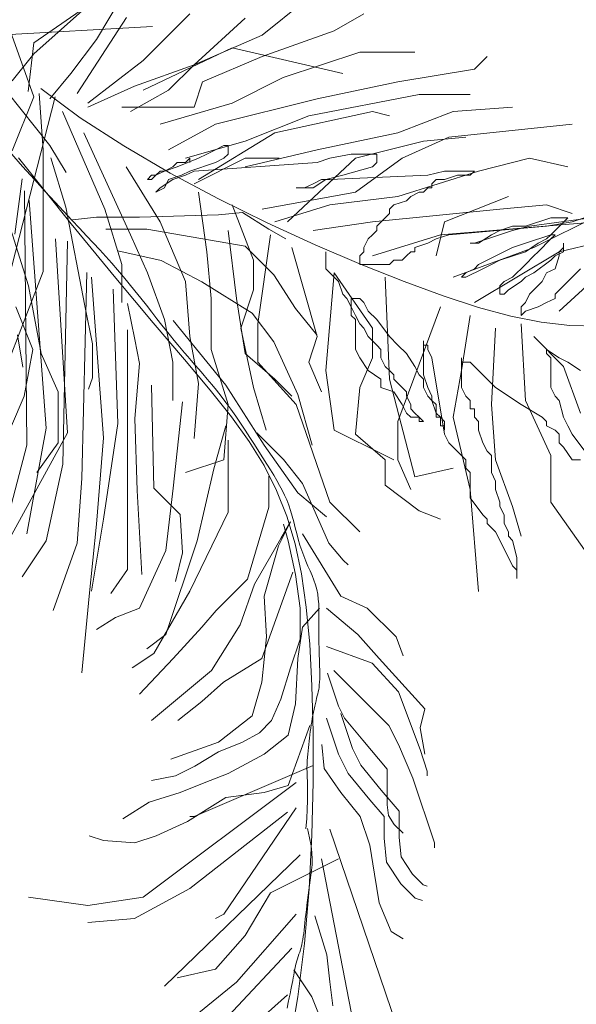
# Model space of a CAD drawing. Units: millimetres. Extents: x 595116 to 630915, y 909473 to 920225.
# Tile 24 of 134: x 629606.562 to 629610.314, y 919164.942 to 919171.576. Entities that reach past the tile are written whole.
import ezdxf

# ---------------------------------------------------------------- set-up
doc = ezdxf.new("R2010")
doc.units = ezdxf.units.MM
doc.layers.add('Dimension', color=3, linetype='Continuous', lineweight=18)
doc.layers.add('L-PLNT', color=85, linetype='Continuous', lineweight=13)
doc.styles.get("Standard").update_dxf_attribs({"font": 'arial.ttf'})
doc.dimstyles.new('ISO-25', dxfattribs={"dimtxt": 9, "dimasz": 6, "dimexe": 1.25, "dimexo": 0.625, "dimtad": 1, "dimlunit": 4, "dimtxsty": 'Standard', "dimcen": 2.5, "dimadec": 0, "dimazin": 0, "dimtfac": 1, "dimtmove": 0, "dimatfit": 3, "dimfxl": 1, "dimarcsym": 0})

# ---------------------------------------------------------------- blocks, each defined once
blk = doc.blocks.new('A$C4FB75ABC')
for p, q in [((2.8539, 2.2576), (2.9801, 2.3449)), ((2.9666, 2.2638), (3.0123, 2.3401)), ((2.8539, 2.2382), (2.9413, 2.3158)), ((3.264, 2.2715), (3.3403, 2.3324)), ((2.9321, 2.167), (3.0207, 2.3031)), ((3.0505, 2.2257), (3.1344, 2.3096)), ((3.142, 2.2181), (3.2335, 2.302)), ((3.3937, 2.2791), (3.447, 2.3096)), ((2.718, 2.2673), (3.0675, 2.2867)), ((2.8054, 2.2964), (2.8539, 2.1606)), ((2.9208, 2.2029), (2.9666, 2.2638)), ((3.142, 2.2181), (3.264, 2.2715)), ((3.264, 2.2334), (3.3937, 2.2791)), ((2.8442, 2.1703), (2.8539, 2.2576)), ((3.0505, 2.1724), (3.2106, 2.2486)), ((3.2106, 2.2486), (3.4089, 2.2029)), ((2.8151, 2.1897), (2.8539, 2.2382)), ((3.1572, 2.1876), (3.264, 2.2334)), ((3.3021, 2.1952), (3.4394, 2.241)), ((3.4394, 2.241), (3.5385, 2.241)), ((3.6453, 2.2105), (3.6682, 2.2334)), ((2.9513, 2.1495), (3.0505, 2.2257)), ((3.0352, 2.18), (3.142, 2.2181)), ((3.0962, 2.1724), (3.142, 2.2181)), ((3.508, 2.1876), (3.6453, 2.2105)), ((2.8827, 2.1571), (2.9208, 2.2029)), ((3.2106, 2.1495), (3.3021, 2.1952)), ((2.9375, 2.1232), (2.8667, 2.1755)), ((2.9513, 2.1419), (3.0352, 2.18)), ((3.142, 2.1419), (3.1572, 2.1876)), ((3.3631, 2.1571), (3.508, 2.1876)), ((2.8927, 2.1606), (2.7957, 1.7822)), ((2.8054, 2.1703), (2.883, 2.0733)), ((2.8539, 2.1606), (2.8151, 2.0636)), ((2.864, 2.167), (2.8708, 2.0648)), ((3.0276, 2.1343), (3.0962, 2.1724)), ((3.1801, 2.1114), (3.3631, 2.1571)), ((3.3479, 2.1266), (3.5462, 2.1648)), ((3.5462, 2.1648), (3.6377, 2.1648)), ((3.0123, 2.1419), (3.142, 2.1419)), ((3.081, 2.1114), (3.2106, 2.1495)), ((3.6072, 2.1343), (3.714, 2.1419)), ((2.9056, 2.1343), (2.9818, 1.9589)), ((3.0158, 2.0725), (2.9375, 2.1232)), ((3.2335, 2.0809), (3.3479, 2.1266)), ((3.2869, 2.0961), (3.4623, 2.1343)), ((3.4623, 2.1343), (3.4928, 2.1266)), ((3.508, 2.0961), (3.6072, 2.1343)), ((3.0962, 2.0657), (3.1801, 2.1114)), ((3.5996, 2.0885), (3.8207, 2.1114)), ((2.9437, 2.0961), (3.0276, 1.9132)), ((3.1496, 2.0123), (3.2869, 2.0961)), ((3.3631, 2.0657), (3.508, 2.0961)), ((3.5157, 2.0504), (3.5996, 2.0885)), ((3.5538, 2.0809), (3.6301, 2.0885)), ((2.883, 2.0733), (2.9122, 2.0248)), ((3.0992, 2.0238), (3.0158, 2.0725)), ((3.1267, 2.0504), (3.2335, 2.0809)), ((3.1954, 2.0733), (3.1801, 2.0657)), ((3.203, 2.0733), (3.1954, 2.0733)), ((3.203, 2.058), (3.203, 2.0733)), ((3.4318, 2.0504), (3.5538, 2.0809)), ((2.8104, 2.0628), (2.8339, 2.0359)), ((2.8268, 2.0511), (2.9214, 1.9326)), ((2.8708, 2.0648), (2.8708, 1.8469)), ((2.8844, 2.0512), (2.9117, 1.9627)), ((3.1496, 2.0504), (3.1115, 2.0352)), ((3.1267, 2.0428), (3.1344, 2.0504)), ((3.1344, 2.0504), (3.1344, 2.0428)), ((3.142, 2.0047), (3.2335, 2.0504)), ((3.1649, 2.058), (3.1496, 2.0504)), ((3.1801, 2.0657), (3.1649, 2.058)), ((3.1801, 2.0428), (3.1954, 2.0504)), ((3.1954, 2.0504), (3.203, 2.058)), ((3.2335, 2.0352), (3.3631, 2.0657)), ((3.2335, 2.0504), (3.2945, 2.0504)), ((3.3098, 1.9361), (3.4318, 2.0504)), ((3.386, 2.0504), (3.3631, 2.0428)), ((3.4242, 2.058), (3.386, 2.0504)), ((3.4699, 2.058), (3.4242, 2.058)), ((3.4318, 1.9894), (3.5157, 2.0504)), ((3.4699, 2.0428), (3.4699, 2.058)), ((3.6529, 2.0275), (3.7445, 2.0504)), ((3.7445, 2.0504), (3.8131, 2.0352)), ((2.8339, 2.0359), (2.8551, 2.0121)), ((3.02, 2.0352), (3.081, 1.9361)), ((3.1115, 2.0352), (3.0886, 2.0275)), ((3.0886, 2.0275), (3.1039, 2.0352)), ((3.1039, 2.0352), (3.1115, 2.0428)), ((3.1115, 2.0428), (3.1267, 2.0428)), ((3.1344, 2.0275), (3.1801, 2.0428)), ((3.3631, 2.0428), (3.142, 2.0275)), ((3.4089, 2.0199), (3.4623, 2.0352)), ((3.4623, 2.0352), (3.4699, 2.0428)), ((3.0581, 2.0123), (3.0657, 2.0199)), ((3.0734, 2.0199), (3.0657, 2.0123)), ((3.0657, 2.0199), (3.0734, 2.0199)), ((3.0734, 2.0199), (3.081, 2.0275)), ((3.0886, 2.0275), (3.0734, 2.0199)), ((3.081, 2.0275), (3.0886, 2.0275)), ((3.0962, 2.0123), (3.1191, 2.0199)), ((3.1858, 1.9776), (3.0992, 2.0238)), ((3.1267, 2.0199), (3.1039, 2.0123)), ((3.1191, 2.0199), (3.1344, 2.0275)), ((3.142, 2.0275), (3.1267, 2.0199)), ((3.3784, 2.0123), (3.4089, 2.0199)), ((3.5614, 2.0199), (3.386, 2.0123)), ((3.508, 1.9818), (3.6529, 2.0275)), ((3.5919, 2.0275), (3.5614, 2.0199)), ((3.6453, 2.0275), (3.5919, 2.0275)), ((3.5919, 2.0123), (3.6148, 2.0199)), ((3.6148, 2.0199), (3.6377, 2.0199)), ((3.6377, 2.0199), (3.6453, 2.0275)), ((2.833, 2.0134), (2.8201, 1.9144)), ((2.8551, 2.0121), (2.8744, 1.9909)), ((3.0657, 2.0123), (3.0581, 2.0123)), ((3.1039, 2.0123), (3.081, 1.9971)), ((3.0886, 1.9971), (3.0962, 2.0123)), ((3.3555, 2.0047), (3.3403, 1.9971)), ((3.3708, 2.0123), (3.3555, 2.0047)), ((3.3555, 1.9971), (3.3784, 2.0123)), ((3.386, 2.0123), (3.3708, 2.0123)), ((3.5691, 2.0047), (3.5767, 2.0123)), ((3.5691, 1.9971), (3.5691, 2.0047)), ((3.5767, 2.0123), (3.5919, 2.0123)), ((2.8373, 1.9919), (2.8416, 1.5357)), ((2.8744, 1.9909), (2.8918, 1.9721)), ((3.081, 1.9971), (3.0734, 1.9894)), ((3.0734, 1.9894), (3.0886, 1.9971)), ((3.1496, 1.9894), (3.1649, 1.8827)), ((3.264, 1.9589), (3.4318, 1.9894)), ((3.3403, 1.9971), (3.325, 1.9971)), ((3.325, 1.9971), (3.3555, 1.9971)), ((3.386, 1.9666), (3.508, 1.9818)), ((3.5233, 1.9742), (3.5309, 1.9818)), ((3.5309, 1.9818), (3.5462, 1.9894)), ((3.5462, 1.9894), (3.5538, 1.9894)), ((3.5538, 1.9894), (3.5614, 1.9971)), ((3.5614, 1.9971), (3.5691, 1.9971)), ((3.5919, 1.9361), (3.7063, 1.9818)), ((2.8459, 1.9747), (2.876, 1.5659)), ((2.8918, 1.9721), (2.9078, 1.955)), ((2.9117, 1.9627), (2.9458, 1.7856)), ((3.2732, 1.9345), (3.1858, 1.9776)), ((3.2106, 1.9666), (3.2488, 1.8675)), ((3.2869, 1.9361), (3.386, 1.9666)), ((3.4928, 1.9589), (3.5004, 1.9666)), ((3.5004, 1.9666), (3.5233, 1.9742)), ((3.6911, 1.9589), (3.775, 1.9666)), ((3.775, 1.9666), (3.8207, 1.9513)), ((2.9078, 1.955), (2.9225, 1.9395)), ((2.9234, 1.9402), (2.9664, 1.9445)), ((2.9664, 1.9445), (3.0439, 1.9445)), ((2.9818, 1.9589), (3.0123, 1.8599)), ((3.0439, 1.9445), (3.186, 1.9488)), ((3.186, 1.9488), (3.2291, 1.9531)), ((3.2291, 1.9531), (3.2764, 1.923)), ((3.4623, 1.9361), (3.6911, 1.9589)), ((3.4852, 1.9437), (3.4928, 1.9513)), ((3.4928, 1.9513), (3.4928, 1.9589)), ((3.7445, 1.9285), (3.9122, 1.9513)), ((3.7521, 1.8903), (3.8894, 1.9589)), ((3.8665, 1.9513), (3.8207, 1.9361)), ((2.8064, 1.9437), (2.8446, 1.8217)), ((2.9214, 1.9326), (3.0014, 1.8351)), ((2.9225, 1.9395), (2.9361, 1.925)), ((3.081, 1.9361), (3.1267, 1.8294)), ((3.3593, 1.8951), (3.2732, 1.9345)), ((3.3555, 1.9208), (3.4623, 1.9361)), ((3.4699, 1.9285), (3.4852, 1.9437)), ((3.4699, 1.9208), (3.4699, 1.9285)), ((3.5767, 1.8751), (3.5919, 1.9361)), ((3.5843, 1.9132), (3.8665, 1.9361)), ((3.775, 1.9285), (3.5996, 1.9132)), ((3.714, 1.9285), (3.6911, 1.9208)), ((3.7368, 1.9285), (3.714, 1.9285)), ((3.714, 1.9208), (3.7445, 1.9285)), ((3.7826, 1.9437), (3.7368, 1.9285)), ((3.8207, 1.9361), (3.775, 1.9285)), ((3.7826, 1.9132), (3.8131, 1.9437)), ((3.8131, 1.9437), (3.7826, 1.9437)), ((3.7978, 1.8827), (4.0495, 1.9437)), ((2.9361, 1.925), (2.9489, 1.9114)), ((2.9489, 1.9114), (2.9609, 1.8985)), ((2.9837, 1.923), (3.0569, 1.923)), ((3.0276, 1.9132), (3.0581, 1.8446)), ((3.0569, 1.923), (3.2334, 1.8929)), ((3.203, 1.9208), (3.2182, 1.7989)), ((3.2793, 1.9132), (3.2564, 1.7531)), ((3.2764, 1.923), (3.3066, 1.9058)), ((3.4547, 1.9056), (3.4623, 1.9132)), ((3.4623, 1.9132), (3.4699, 1.9208)), ((3.4623, 1.8751), (3.5843, 1.9132)), ((3.5996, 1.9132), (3.5767, 1.9056)), ((3.6453, 1.898), (3.714, 1.9208)), ((3.6758, 1.9132), (3.6529, 1.898)), ((3.6911, 1.9208), (3.6758, 1.9132)), ((3.7368, 1.898), (3.7826, 1.9132)), ((3.7826, 1.9132), (3.775, 1.9056)), ((3.7826, 1.9056), (3.7902, 1.9132)), ((3.7902, 1.9132), (3.7826, 1.9132)), ((2.8933, 1.9058), (2.9148, 1.5573)), ((2.9148, 1.9015), (2.9062, 1.5013)), ((2.9609, 1.8985), (2.9724, 1.8861)), ((3.2334, 1.8929), (3.285, 1.8413)), ((3.4421, 1.8597), (3.3593, 1.8951)), ((3.447, 1.8903), (3.4547, 1.9056)), ((3.5614, 1.898), (3.5385, 1.8903)), ((3.5767, 1.9056), (3.5614, 1.898)), ((3.6529, 1.898), (3.6377, 1.898)), ((3.6377, 1.898), (3.6453, 1.898)), ((3.714, 1.8903), (3.7368, 1.898)), ((3.7597, 1.898), (3.7368, 1.8827)), ((3.7597, 1.8827), (3.7826, 1.9056)), ((3.775, 1.9056), (3.7597, 1.898)), ((3.8055, 1.8903), (3.8055, 1.898)), ((3.8055, 1.898), (3.8055, 1.8827)), ((2.9724, 1.8861), (2.9834, 1.874)), ((2.9834, 1.874), (2.994, 1.862)), ((3.0052, 1.8843), (3.0827, 1.8671)), ((3.1649, 1.8827), (3.1725, 1.7989)), ((3.3174, 1.8903), (3.3631, 1.7303)), ((3.3784, 1.8827), (3.3784, 1.8522)), ((3.4394, 1.8751), (3.447, 1.8827)), ((3.4394, 1.8599), (3.4394, 1.8751)), ((3.447, 1.8827), (3.447, 1.8903)), ((3.5233, 1.8751), (3.5157, 1.8675)), ((3.5309, 1.8827), (3.5233, 1.8751)), ((3.5385, 1.8827), (3.5309, 1.8827)), ((3.5385, 1.8903), (3.5385, 1.8827)), ((3.6072, 1.837), (3.7521, 1.8903)), ((3.6453, 1.7913), (3.7978, 1.8827)), ((3.6682, 1.8675), (3.714, 1.8903)), ((3.7368, 1.8827), (3.6911, 1.8675)), ((3.7368, 1.8599), (3.7521, 1.8751)), ((3.7521, 1.8751), (3.7597, 1.8827)), ((3.7902, 1.8751), (3.7826, 1.8675)), ((3.8055, 1.8827), (3.7902, 1.8751)), ((3.7902, 1.8522), (3.7978, 1.8751)), ((3.7978, 1.8827), (3.8055, 1.8903)), ((3.7978, 1.8751), (3.7978, 1.8827)), ((2.994, 1.862), (3.0045, 1.8499)), ((3.0123, 1.8599), (3.0123, 1.7913)), ((3.0827, 1.8671), (3.1559, 1.8284)), ((3.2488, 1.8675), (3.2488, 1.8141)), ((3.4928, 1.8599), (3.4394, 1.8599)), ((3.5192, 1.829), (3.4421, 1.8597)), ((3.5004, 1.8675), (3.4928, 1.8599)), ((3.5157, 1.8675), (3.5004, 1.8675)), ((3.6453, 1.8522), (3.6529, 1.8599)), ((3.6529, 1.8599), (3.6682, 1.8675)), ((3.6758, 1.8599), (3.6606, 1.8522)), ((3.6911, 1.8675), (3.6758, 1.8599)), ((3.714, 1.837), (3.7368, 1.8599)), ((3.7826, 1.8675), (3.7521, 1.8446)), ((3.7978, 1.776), (3.897, 1.8675)), ((2.8708, 1.8469), (2.8027, 1.6699)), ((2.9492, 1.8456), (2.9406, 1.4755)), ((3.0045, 1.8499), (3.0149, 1.8377)), ((3.0581, 1.8446), (3.0886, 1.7608)), ((3.285, 1.8413), (3.3238, 1.781)), ((3.3784, 1.8522), (3.3937, 1.837)), ((3.3937, 1.8446), (3.3784, 1.6693)), ((3.3937, 1.8446), (3.4623, 1.7455)), ((3.6224, 1.837), (3.6301, 1.8446)), ((3.6606, 1.8522), (3.6301, 1.837)), ((3.6301, 1.8446), (3.6453, 1.8522)), ((3.7521, 1.8446), (3.7368, 1.837)), ((3.7673, 1.8294), (3.775, 1.8446)), ((3.775, 1.8446), (3.7902, 1.8522)), ((3.836, 1.8522), (3.8207, 1.837)), ((2.8446, 1.8217), (2.8674, 1.6998)), ((2.9578, 1.837), (2.9794, 1.5486)), ((3.0014, 1.8351), (3.0686, 1.7552)), ((3.0149, 1.8377), (3.0253, 1.8251)), ((3.0253, 1.8251), (3.0358, 1.8122)), ((3.1267, 1.8294), (3.1344, 1.7303)), ((3.1559, 1.8284), (3.2463, 1.7724)), ((3.3937, 1.837), (3.4013, 1.8294)), ((3.4013, 1.8294), (3.4089, 1.8065)), ((3.4852, 1.837), (3.4928, 1.6541)), ((3.5892, 1.8034), (3.5192, 1.829)), ((3.6301, 1.837), (3.6224, 1.837)), ((3.6911, 1.8217), (3.6987, 1.8294)), ((3.6911, 1.8065), (3.6911, 1.8217)), ((3.6987, 1.8294), (3.714, 1.837)), ((3.7292, 1.8294), (3.7063, 1.8141)), ((3.7368, 1.837), (3.7292, 1.8294)), ((3.7445, 1.8065), (3.7673, 1.8294)), ((3.8131, 1.8294), (3.7902, 1.8065)), ((3.8207, 1.837), (3.8131, 1.8294)), ((2.9966, 1.8154), (3.0052, 1.5745)), ((3.0358, 1.8122), (3.0461, 1.7993)), ((3.2488, 1.8141), (3.2259, 1.7455)), ((3.4089, 1.8065), (3.4165, 1.7989)), ((3.6527, 1.7828), (3.5892, 1.8034)), ((3.6987, 1.8065), (3.6911, 1.8065)), ((3.7063, 1.8141), (3.6987, 1.8065)), ((3.7368, 1.7913), (3.7445, 1.8065)), ((3.7902, 1.8065), (3.7902, 1.7989)), ((2.9458, 1.7856), (2.9594, 1.7175)), ((3.0224, 1.7896), (3.0353, 1.7251)), ((3.0461, 1.7993), (3.0562, 1.7866)), ((3.0562, 1.7866), (3.0659, 1.7741)), ((3.1725, 1.7989), (3.1725, 1.7074)), ((3.2182, 1.7989), (3.2335, 1.6998)), ((3.4165, 1.7989), (3.4242, 1.7836)), ((3.4242, 1.7684), (3.4242, 1.7989)), ((3.4242, 1.7989), (3.4394, 1.7989)), ((3.4394, 1.7989), (3.447, 1.7913)), ((3.447, 1.7913), (3.4547, 1.776)), ((3.7292, 1.7836), (3.7368, 1.7913)), ((3.775, 1.7913), (3.7597, 1.7836)), ((3.7902, 1.7989), (3.775, 1.7913)), ((2.8217, 1.7836), (2.8522, 1.7074)), ((3.0659, 1.7741), (3.0752, 1.7623)), ((3.2463, 1.7724), (3.285, 1.7208)), ((3.3238, 1.781), (3.3625, 1.7337)), ((3.4242, 1.7836), (3.4318, 1.7684)), ((3.4318, 1.7608), (3.4242, 1.7684)), ((3.4318, 1.7684), (3.4394, 1.7531)), ((3.4547, 1.776), (3.4699, 1.7608)), ((3.5843, 1.7836), (3.508, 1.5778)), ((3.6377, 1.7684), (3.6224, 1.6693)), ((3.7109, 1.7672), (3.6527, 1.7828)), ((3.7292, 1.7684), (3.7292, 1.7836)), ((3.7368, 1.776), (3.7292, 1.7684)), ((3.7597, 1.7836), (3.7368, 1.776)), ((3.0686, 1.7552), (3.1246, 1.6894)), ((3.0752, 1.7623), (3.084, 1.7511)), ((3.084, 1.7511), (3.0921, 1.7408)), ((3.0886, 1.7608), (3.1039, 1.6845)), ((3.1042, 1.7595), (3.1989, 1.6433)), ((3.2564, 1.7531), (3.2564, 1.6845)), ((3.4318, 1.7074), (3.4318, 1.7608)), ((3.4394, 1.7531), (3.447, 1.7455)), ((3.4699, 1.7608), (3.4928, 1.7303)), ((3.7651, 1.7564), (3.7109, 1.7672)), ((3.7292, 1.7531), (3.7368, 1.6159)), ((3.8165, 1.7504), (3.7651, 1.7564)), ((3.8664, 1.749), (3.8165, 1.7504)), ((2.8248, 1.7337), (2.8345, 1.6755)), ((3.0224, 1.7423), (3.0224, 1.312)), ((3.0921, 1.7408), (3.0994, 1.7316)), ((3.2259, 1.7455), (3.2488, 1.6388)), ((3.447, 1.7455), (3.4547, 1.7303)), ((3.4623, 1.7455), (3.4623, 1.6922)), ((3.6834, 1.7455), (3.6758, 1.6083)), ((2.9594, 1.7175), (2.9594, 1.6563)), ((3.0353, 1.7251), (3.0439, 1.682)), ((3.0994, 1.7316), (3.1062, 1.7232)), ((3.1062, 1.7232), (3.1126, 1.7155)), ((3.1126, 1.7155), (3.1186, 1.7083)), ((3.1344, 1.7303), (3.1496, 1.6464)), ((3.285, 1.7208), (3.3281, 1.6261)), ((3.3631, 1.7303), (3.3479, 1.6845)), ((3.4547, 1.7303), (3.4699, 1.715)), ((3.4699, 1.715), (3.4775, 1.7074)), ((3.4928, 1.7303), (3.508, 1.715)), ((3.508, 1.715), (3.5233, 1.6998)), ((3.5538, 1.7227), (3.5538, 1.715)), ((3.5538, 1.6617), (3.5538, 1.7227)), ((3.5538, 1.715), (3.5614, 1.715)), ((3.5614, 1.715), (3.5614, 1.7074)), ((3.7521, 1.7303), (3.8055, 1.6769)), ((2.8522, 1.7074), (2.8369, 1.6236)), ((2.8674, 1.6998), (2.8979, 1.6312)), ((3.1186, 1.7083), (3.1246, 1.7013)), ((3.1246, 1.7013), (3.1305, 1.6944)), ((3.1725, 1.7074), (3.203, 1.6083)), ((3.2335, 1.6998), (3.2869, 1.6541)), ((3.4394, 1.6922), (3.4318, 1.7074)), ((3.4775, 1.7074), (3.4775, 1.6922)), ((3.5233, 1.6998), (3.5385, 1.6769)), ((3.5614, 1.7074), (3.5691, 1.6922)), ((3.775, 1.6998), (3.775, 1.7074)), ((3.775, 1.7074), (3.7978, 1.6922)), ((3.7826, 1.6922), (3.775, 1.6998)), ((3.0439, 1.682), (3.0353, 1.5831)), ((3.1039, 1.6845), (3.1039, 1.6159)), ((3.1246, 1.6894), (3.1709, 1.6342)), ((3.1305, 1.6944), (3.1367, 1.6873)), ((3.1367, 1.6873), (3.1432, 1.6798)), ((3.1432, 1.6798), (3.1502, 1.6718)), ((3.2564, 1.6845), (3.325, 1.6083)), ((3.3479, 1.6845), (3.3708, 1.6312)), ((3.4547, 1.6693), (3.4394, 1.6922)), ((3.4623, 1.6922), (3.4394, 1.6388)), ((3.4775, 1.6922), (3.4852, 1.6769)), ((3.5691, 1.6922), (3.5919, 1.555)), ((3.6224, 1.6922), (3.6224, 1.6845)), ((3.6224, 1.6388), (3.6224, 1.6922)), ((3.6224, 1.6845), (3.6377, 1.6845)), ((3.6377, 1.6845), (3.6453, 1.6769)), ((3.7826, 1.6388), (3.7826, 1.6922)), ((3.7978, 1.6922), (3.8131, 1.6845)), ((3.8131, 1.6845), (3.836, 1.6693)), ((3.1502, 1.6718), (3.1576, 1.6632)), ((3.1576, 1.6632), (3.1654, 1.654)), ((3.3784, 1.6693), (3.3937, 1.5626)), ((3.4775, 1.6541), (3.4547, 1.6693)), ((3.4852, 1.6769), (3.4928, 1.6693)), ((3.4928, 1.6693), (3.5004, 1.6617)), ((3.5004, 1.6617), (3.5004, 1.6541)), ((3.5385, 1.6769), (3.5462, 1.6617)), ((3.5462, 1.6617), (3.5538, 1.6541)), ((3.5614, 1.6388), (3.5538, 1.6617)), ((3.6224, 1.6693), (3.6072, 1.5855)), ((3.6453, 1.6769), (3.6682, 1.6541)), ((3.8055, 1.6769), (3.836, 1.5931)), ((2.9594, 1.6563), (2.9526, 1.6358)), ((3.1496, 1.6464), (3.142, 1.5473)), ((3.1654, 1.654), (3.1735, 1.6443)), ((3.1735, 1.6443), (3.1819, 1.634)), ((3.2869, 1.6541), (3.3174, 1.6236)), ((3.4775, 1.6388), (3.4775, 1.6541)), ((3.4928, 1.6541), (3.5385, 1.4787)), ((3.5004, 1.6541), (3.5157, 1.6388)), ((3.5538, 1.6541), (3.5538, 1.6388)), ((3.6682, 1.6541), (3.6834, 1.6388)), ((2.8979, 1.6312), (2.8979, 1.5397)), ((3.0655, 1.6433), (3.0698, 1.4583)), ((3.1709, 1.6342), (3.2091, 1.5863)), ((3.1819, 1.634), (3.1904, 1.6232)), ((3.1989, 1.6433), (3.2678, 1.5357)), ((3.2488, 1.6388), (3.2716, 1.5626)), ((3.3281, 1.6261), (3.3539, 1.5357)), ((3.4394, 1.6388), (3.4318, 1.555)), ((3.5004, 1.6312), (3.4775, 1.6388)), ((3.5157, 1.6083), (3.5004, 1.6312)), ((3.5157, 1.6388), (3.5233, 1.6312)), ((3.5233, 1.6312), (3.5233, 1.6236)), ((3.5538, 1.6388), (3.5614, 1.6236)), ((3.5691, 1.6236), (3.5614, 1.6388)), ((3.6301, 1.6236), (3.6224, 1.6388)), ((3.6834, 1.6388), (3.7292, 1.6083)), ((3.7902, 1.6236), (3.7826, 1.6388)), ((2.8369, 1.6236), (2.8141, 1.5702)), ((3.1214, 1.6132), (3.1042, 1.4583)), ((3.1904, 1.6232), (3.1991, 1.6119)), ((3.1991, 1.6119), (3.2078, 1.6)), ((3.5233, 1.6236), (3.5309, 1.6083)), ((3.5614, 1.6236), (3.5691, 1.6159)), ((3.5691, 1.6159), (3.5691, 1.6236)), ((3.5691, 1.6159), (3.5767, 1.6083)), ((3.5767, 1.5931), (3.5691, 1.6159)), ((3.6377, 1.6159), (3.6301, 1.6236)), ((3.6377, 1.6007), (3.6377, 1.6159)), ((3.7368, 1.6159), (3.7826, 1.5168)), ((3.7978, 1.6159), (3.7902, 1.6236)), ((3.8055, 1.5855), (3.7978, 1.6159)), ((3.203, 1.6083), (3.1954, 1.5092)), ((3.2078, 1.6), (3.2166, 1.5877)), ((3.325, 1.6083), (3.386, 1.433)), ((3.5233, 1.5931), (3.5157, 1.6083)), ((3.5309, 1.5855), (3.5233, 1.5931)), ((3.5309, 1.6083), (3.5309, 1.6007)), ((3.5309, 1.6007), (3.5385, 1.5931)), ((3.5385, 1.5931), (3.5462, 1.5855)), ((3.5767, 1.6083), (3.5767, 1.5855)), ((3.5843, 1.5855), (3.5767, 1.5931)), ((3.6453, 1.6007), (3.6377, 1.6007)), ((3.6453, 1.5855), (3.6453, 1.6007)), ((3.6758, 1.6083), (3.6834, 1.5092)), ((3.7292, 1.6083), (3.7673, 1.5855)), ((3.0052, 1.5745), (2.9794, 1.4023)), ((3.0353, 1.5831), (3.0396, 1.454)), ((3.2091, 1.5863), (3.241, 1.5422)), ((3.2166, 1.5877), (3.2252, 1.575)), ((3.2252, 1.575), (3.2338, 1.5622)), ((3.508, 1.5778), (3.508, 1.5092)), ((3.5462, 1.5855), (3.5309, 1.5855)), ((3.5462, 1.5855), (3.5462, 1.5778)), ((3.5538, 1.5778), (3.5462, 1.5855)), ((3.5462, 1.5778), (3.5538, 1.5778)), ((3.5767, 1.5855), (3.5843, 1.5855)), ((3.5843, 1.5855), (3.5843, 1.5702)), ((3.5919, 1.5778), (3.5843, 1.5855)), ((3.5919, 1.5626), (3.5919, 1.5778)), ((3.6072, 1.5855), (3.6377, 1.4559)), ((3.6529, 1.5778), (3.6453, 1.5855)), ((3.6529, 1.5626), (3.6529, 1.5778)), ((3.7673, 1.5855), (3.775, 1.5778)), ((3.775, 1.5778), (3.775, 1.5702)), ((3.8131, 1.5702), (3.8055, 1.5855)), ((2.9148, 1.5573), (2.7942, 1.3378)), ((2.876, 1.5659), (2.8416, 1.3765)), ((3.1989, 1.5702), (3.1774, 1.4927)), ((3.2338, 1.5622), (3.2421, 1.5493)), ((3.2549, 1.5573), (3.3023, 1.5099)), ((3.3937, 1.5626), (3.4852, 1.5168)), ((3.5843, 1.5702), (3.5919, 1.5702)), ((3.5919, 1.5702), (3.5919, 1.5626)), ((3.6606, 1.5397), (3.6529, 1.5626)), ((3.775, 1.5702), (3.7902, 1.5626)), ((3.7902, 1.5626), (3.7978, 1.555)), ((3.8207, 1.555), (3.8131, 1.5702)), ((2.8979, 1.5397), (2.8598, 1.4864)), ((2.9794, 1.5486), (2.9664, 1.3937)), ((3.2032, 1.5443), (3.2032, 1.4152)), ((3.241, 1.5422), (3.2678, 1.4987)), ((3.2421, 1.5493), (3.2503, 1.5367)), ((3.4318, 1.555), (3.4852, 1.5092)), ((3.5919, 1.555), (3.5996, 1.5397)), ((3.5996, 1.5397), (3.6301, 1.5092)), ((3.6682, 1.5245), (3.6606, 1.5397)), ((3.7978, 1.555), (3.7978, 1.5397)), ((3.7978, 1.5397), (3.8055, 1.5321)), ((3.8436, 1.5245), (3.8207, 1.555)), ((2.8416, 1.5357), (2.8071, 1.4023)), ((3.2503, 1.5367), (3.258, 1.5243)), ((3.258, 1.5243), (3.2655, 1.5125)), ((3.2678, 1.5357), (3.3281, 1.4497)), ((3.6758, 1.5168), (3.6682, 1.5245)), ((3.8055, 1.5321), (3.8207, 1.5092)), ((3.1954, 1.5092), (3.1267, 1.4864)), ((3.2655, 1.5125), (3.2724, 1.5013)), ((3.3023, 1.5099), (3.3367, 1.4669)), ((3.4852, 1.5168), (3.5004, 1.5092)), ((3.4852, 1.5092), (3.4852, 1.4635)), ((3.508, 1.5092), (3.5309, 1.4559)), ((3.6301, 1.5092), (3.6301, 1.494)), ((3.6758, 1.4864), (3.6758, 1.5168)), ((3.6834, 1.5092), (3.714, 1.4254)), ((3.7826, 1.5168), (3.7826, 1.433)), ((3.8207, 1.5092), (3.836, 1.5092)), ((2.9062, 1.5013), (2.876, 1.3636)), ((3.1774, 1.4927), (3.1473, 1.3636)), ((3.2678, 1.4987), (3.2902, 1.4543)), ((3.2724, 1.5013), (3.2789, 1.491)), ((3.2789, 1.491), (3.2849, 1.4813)), ((3.5385, 1.4787), (3.6072, 1.494)), ((3.6301, 1.494), (3.6377, 1.4864)), ((3.6377, 1.4864), (3.6377, 1.4406)), ((3.6834, 1.4711), (3.6758, 1.4864)), ((2.9406, 1.4755), (2.932, 1.3593)), ((3.2764, 1.4798), (3.2764, 1.4239)), ((3.2849, 1.4813), (3.2904, 1.4721)), ((3.2904, 1.4721), (3.2955, 1.4632)), ((3.6834, 1.4559), (3.6834, 1.4711)), ((3.0396, 1.454), (3.0483, 1.3034)), ((3.0698, 1.4583), (3.1171, 1.4109)), ((3.1042, 1.4583), (3.0913, 1.3464)), ((3.2902, 1.4543), (3.3086, 1.4079)), ((3.2955, 1.4632), (3.3002, 1.4545)), ((3.3002, 1.4545), (3.3045, 1.4458)), ((3.3281, 1.4497), (3.3798, 1.4066)), ((3.3367, 1.4669), (3.3841, 1.3593)), ((3.4852, 1.4635), (3.5462, 1.4178)), ((3.6377, 1.4559), (3.6529, 1.2729)), ((3.6911, 1.433), (3.6834, 1.4559)), ((3.3045, 1.4458), (3.3084, 1.437)), ((3.3084, 1.437), (3.3119, 1.4278)), ((3.386, 1.433), (3.4394, 1.3796)), ((3.6377, 1.4406), (3.6606, 1.4101)), ((3.6911, 1.4254), (3.6911, 1.433)), ((3.7826, 1.433), (3.8741, 1.3034)), ((3.2032, 1.4152), (3.1344, 1.2732)), ((3.2764, 1.4239), (3.2377, 1.2948)), ((3.3119, 1.4278), (3.3151, 1.4181)), ((3.3151, 1.4181), (3.3181, 1.4081)), ((3.5462, 1.4178), (3.5843, 1.4025)), ((3.6987, 1.4101), (3.6911, 1.4254)), ((3.714, 1.4254), (3.7292, 1.372)), ((2.9794, 1.4023), (2.9578, 1.2732)), ((3.1171, 1.4109), (3.1214, 1.3421)), ((3.2937, 1.355), (3.3152, 1.398)), ((3.298, 1.3679), (3.3152, 1.398)), ((3.3086, 1.4079), (3.3233, 1.3583)), ((3.3181, 1.4081), (3.3209, 1.3978)), ((3.3209, 1.3978), (3.3236, 1.3873)), ((3.6606, 1.4101), (3.6682, 1.4025)), ((3.6682, 1.4025), (3.6682, 1.3949)), ((3.6987, 1.3949), (3.6987, 1.4101)), ((2.9664, 1.3937), (2.9535, 1.2646)), ((3.3023, 1.3937), (3.3109, 1.3636)), ((3.3236, 1.3873), (3.3263, 1.3768)), ((3.6682, 1.3949), (3.6834, 1.3796)), ((3.6834, 1.3796), (3.6987, 1.3492)), ((3.7063, 1.3796), (3.6987, 1.3949)), ((3.7063, 1.372), (3.7063, 1.3796)), ((2.876, 1.3636), (2.833, 1.2991)), ((3.1473, 1.3636), (3.0913, 1.1958)), ((3.2506, 1.2861), (3.298, 1.3679)), ((3.3109, 1.3636), (3.3238, 1.3034)), ((3.3263, 1.3768), (3.3291, 1.3664)), ((3.3291, 1.3664), (3.332, 1.3561)), ((3.3367, 1.3765), (3.4056, 1.2646)), ((3.714, 1.3644), (3.7063, 1.372)), ((3.7216, 1.3339), (3.714, 1.3644)), ((2.932, 1.3593), (2.889, 1.2388)), ((3.0913, 1.3464), (3.0439, 1.2431)), ((3.2678, 1.2646), (3.2937, 1.355)), ((3.3233, 1.3583), (3.3348, 1.3042)), ((3.332, 1.3561), (3.3352, 1.3462)), ((3.3352, 1.3462), (3.3388, 1.3366)), ((3.3841, 1.3593), (3.4099, 1.3292)), ((3.6987, 1.3492), (3.714, 1.3187)), ((3.1214, 1.3421), (3.1085, 1.2905)), ((3.3388, 1.3366), (3.3425, 1.3274)), ((3.3425, 1.3274), (3.3463, 1.3185)), ((3.4099, 1.3292), (3.4185, 1.3206)), ((3.7216, 1.2958), (3.7216, 1.3339)), ((3.0224, 1.312), (2.9923, 1.2689)), ((3.3463, 1.3185), (3.3501, 1.3098)), ((3.3501, 1.3098), (3.3537, 1.3013)), ((3.714, 1.3187), (3.7216, 1.311)), ((3.7216, 1.311), (3.7216, 1.2958)), ((3.2377, 1.2948), (3.1817, 1.2388)), ((3.3195, 1.3077), (3.2635, 1.1527)), ((3.3238, 1.3034), (3.3324, 1.2431)), ((3.3348, 1.3042), (3.3434, 1.2446)), ((3.3537, 1.3013), (3.357, 1.2929)), ((3.357, 1.2929), (3.3598, 1.2846)), ((3.1344, 1.2732), (3.0698, 1.1614)), ((3.2248, 1.213), (3.2506, 1.2861)), ((3.3598, 1.2846), (3.3622, 1.2762)), ((3.3622, 1.2762), (3.3639, 1.2677)), ((2.9535, 1.2646), (2.9406, 1.1269)), ((3.2721, 1.1915), (3.2678, 1.2646)), ((3.3639, 1.2677), (3.365, 1.2592)), ((3.365, 1.2592), (3.3657, 1.2504)), ((3.4056, 1.2646), (3.453, 1.2431)), ((3.0439, 1.2431), (3.0009, 1.2259)), ((3.1817, 1.2388), (3.1559, 1.2087)), ((3.3324, 1.2431), (3.3324, 1.1872)), ((3.3367, 1.2087), (3.3669, 1.2431)), ((3.3434, 1.2446), (3.3495, 1.1781)), ((3.3657, 1.2504), (3.366, 1.2415)), ((3.366, 1.2415), (3.366, 1.2322)), ((3.3798, 1.2431), (3.4357, 1.1958)), ((3.453, 1.2431), (3.5046, 1.1915)), ((3.0009, 1.2259), (2.9664, 1.2044)), ((3.366, 1.2227), (3.3658, 1.2129)), ((3.366, 1.2322), (3.366, 1.2227)), ((3.1559, 1.2087), (3.1042, 1.1527)), ((3.1731, 1.1312), (3.2248, 1.213)), ((3.3281, 1.1527), (3.3367, 1.2087)), ((3.3658, 1.2129), (3.3658, 1.2027)), ((3.3658, 1.2027), (3.3658, 1.1921)), ((3.0913, 1.1958), (3.0569, 1.17)), ((3.2635, 1.1097), (3.2721, 1.1915)), ((3.3324, 1.1872), (3.3152, 1.1355)), ((3.3658, 1.1921), (3.366, 1.1812)), ((3.4357, 1.1958), (3.4745, 1.1527)), ((3.5046, 1.1915), (3.5175, 1.1571)), ((3.3495, 1.1781), (3.3535, 1.1037)), ((3.366, 1.1812), (3.3663, 1.1704)), ((3.3663, 1.1704), (3.3667, 1.1597)), ((3.3798, 1.1743), (3.4616, 1.1441)), ((3.0698, 1.1614), (3.031, 1.1355)), ((3.1042, 1.1527), (3.0439, 1.0882)), ((3.2635, 1.1527), (3.1946, 1.1097)), ((3.3238, 1.071), (3.3281, 1.1527)), ((3.3667, 1.1597), (3.367, 1.1494)), ((3.367, 1.1494), (3.3673, 1.1397)), ((3.4745, 1.1527), (3.5563, 1.0624)), ((3.0655, 1.0409), (3.1731, 1.1312)), ((3.3152, 1.1355), (3.298, 1.0796)), ((3.3673, 1.1397), (3.3675, 1.1308)), ((3.3927, 1.1312), (3.44, 1.0839)), ((3.4616, 1.1441), (3.5089, 1.0925)), ((3.3675, 1.116), (3.3672, 1.1101)), ((3.3675, 1.1308), (3.3676, 1.1228)), ((3.3676, 1.1228), (3.3675, 1.116)), ((3.3816, 1.1261), (3.4013, 1.0669)), ((3.1946, 1.1097), (3.1559, 1.0753)), ((3.2463, 1.0495), (3.2635, 1.1097)), ((3.3535, 1.1037), (3.3557, 1.0207)), ((3.3657, 1.0966), (3.3649, 1.0928)), ((3.3663, 1.1006), (3.3657, 1.0966)), ((3.3668, 1.1051), (3.3663, 1.1006)), ((3.3672, 1.1101), (3.3668, 1.1051)), ((3.298, 1.0796), (3.2807, 1.0409)), ((3.362, 1.081), (3.3609, 1.0765)), ((3.3631, 1.0852), (3.362, 1.081)), ((3.364, 1.0891), (3.3631, 1.0852)), ((3.3649, 1.0928), (3.364, 1.0891)), ((3.44, 1.0839), (3.4917, 1.0323)), ((3.5089, 1.0925), (3.5477, 0.9892)), ((3.1559, 1.0753), (3.1128, 1.0409)), ((3.3109, 1.015), (3.3238, 1.071)), ((3.3574, 1.0614), (3.3563, 1.056)), ((3.3586, 1.0667), (3.3574, 1.0614)), ((3.3598, 1.0717), (3.3586, 1.0667)), ((3.3609, 1.0765), (3.3598, 1.0717)), ((3.4013, 1.0669), (3.4121, 1.0454)), ((3.5563, 1.0624), (3.5477, 1.028)), ((3.186, 1.0021), (3.2463, 1.0495)), ((3.3541, 1.0448), (3.3531, 1.039)), ((3.3551, 1.0505), (3.3541, 1.0448)), ((3.3563, 1.056), (3.3551, 1.0505)), ((3.3798, 1.0452), (3.4013, 0.9806)), ((3.4053, 1.0537), (3.4263, 0.991)), ((3.4121, 1.0454), (3.4447, 1.0056)), ((3.2807, 1.0409), (3.2592, 1.0193)), ((3.3496, 1.0323), (3.3109, 0.9247)), ((3.3514, 1.0274), (3.3506, 1.0215)), ((3.3522, 1.0332), (3.3514, 1.0274)), ((3.3531, 1.039), (3.3522, 1.0332)), ((3.4917, 1.0323), (3.5089, 0.9978)), ((3.5477, 1.028), (3.5563, 0.9806)), ((3.2592, 1.0193), (3.2291, 1.0021)), ((3.2678, 0.9806), (3.3109, 1.015)), ((3.3492, 1.0097), (3.3485, 1.0039)), ((3.3499, 1.0156), (3.3492, 1.0097)), ((3.3506, 1.0215), (3.3499, 1.0156)), ((3.3557, 1.0207), (3.3558, 0.9307)), ((3.0999, 0.972), (3.186, 1.0021)), ((3.2291, 1.0021), (3.186, 0.9849)), ((3.3471, 0.9925), (3.3465, 0.9868)), ((3.3478, 0.9982), (3.3471, 0.9925)), ((3.3485, 1.0039), (3.3478, 0.9982)), ((3.3712, 0.9978), (3.3755, 0.9548)), ((3.4263, 0.991), (3.4413, 0.9609)), ((3.4447, 1.0056), (3.4889, 0.9539)), ((3.5089, 0.9978), (3.5348, 0.9376)), ((3.186, 0.9849), (3.143, 0.9591)), ((3.2032, 0.9462), (3.2678, 0.9806)), ((3.3454, 0.9751), (3.345, 0.9689)), ((3.3459, 0.981), (3.3454, 0.9751)), ((3.3465, 0.9868), (3.3459, 0.981)), ((3.4013, 0.9806), (3.4185, 0.9462)), ((3.5477, 0.9892), (3.5606, 0.9505)), ((3.143, 0.9591), (3.1085, 0.9419)), ((3.3555, 0.9604), (3.142, 0.8689)), ((3.3447, 0.9623), (3.3446, 0.9554)), ((3.3446, 0.9554), (3.3447, 0.9479)), ((3.345, 0.9689), (3.3447, 0.9623)), ((3.3755, 0.9548), (3.4056, 0.9118)), ((3.4413, 0.9609), (3.4779, 0.9162)), ((3.1085, 0.9419), (3.0655, 0.9333)), ((3.1602, 0.929), (3.2032, 0.9462)), ((3.3447, 0.9479), (3.3449, 0.9399)), ((3.3449, 0.9399), (3.3453, 0.931)), ((3.4185, 0.9462), (3.4573, 0.8989)), ((3.4889, 0.9539), (3.4889, 0.8899)), ((3.5348, 0.9376), (3.5735, 0.8214)), ((3.5606, 0.9505), (3.5606, 0.9419)), ((3.325, 0.9299), (3.0505, 0.7241)), ((3.1171, 0.9118), (3.1602, 0.929)), ((3.3109, 0.9247), (3.2678, 0.9118)), ((3.3453, 0.931), (3.3456, 0.921)), ((3.3456, 0.921), (3.3457, 0.9097)), ((3.3558, 0.9307), (3.3535, 0.836)), ((3.0612, 0.8946), (3.1171, 0.9118)), ((3.1989, 0.9032), (3.1301, 0.8601)), ((3.2678, 0.9118), (3.1989, 0.9032)), ((3.3457, 0.9097), (3.3456, 0.8969)), ((3.4056, 0.9118), (3.44, 0.8687)), ((3.4779, 0.9162), (3.5101, 0.8787)), ((3.0138, 0.8644), (3.0612, 0.8946)), ((3.325, 0.8842), (3.1954, 0.6936)), ((3.3456, 0.8969), (3.3451, 0.8822)), ((3.4573, 0.8989), (3.4831, 0.8687)), ((3.4889, 0.8899), (3.4909, 0.8704)), ((3.3098, 0.8766), (3.1344, 0.7394)), ((3.142, 0.8689), (3.1344, 0.8689)), ((3.3451, 0.8822), (3.3441, 0.8655)), ((3.44, 0.8687), (3.4573, 0.8171)), ((3.4831, 0.8687), (3.4831, 0.83)), ((3.4909, 0.8704), (3.5015, 0.8546)), ((3.5101, 0.8787), (3.5101, 0.8314)), ((3.1301, 0.8601), (3.0741, 0.8343)), ((3.3441, 0.8655), (3.3424, 0.8466)), ((3.5015, 0.8546), (3.5172, 0.8388)), ((2.9794, 0.8257), (2.9535, 0.8343)), ((3.0741, 0.8343), (3.0353, 0.8214)), ((3.3453, 0.8472), (3.3494, 0.8306)), ((3.3535, 0.836), (3.3484, 0.7387)), ((3.386, 0.8461), (3.508, 0.4878)), ((3.5101, 0.8314), (3.5136, 0.7963)), ((3.0353, 0.8214), (2.9794, 0.8257)), ((3.3494, 0.8306), (3.3521, 0.8161)), ((3.3521, 0.8161), (3.3535, 0.8034)), ((3.4573, 0.8171), (3.4659, 0.7655)), ((3.4831, 0.83), (3.4874, 0.787)), ((3.5735, 0.8214), (3.5735, 0.8128)), ((3.3326, 0.8003), (3.0886, 0.5641)), ((3.3535, 0.8034), (3.354, 0.7921)), ((3.5136, 0.7963), (3.5342, 0.7654)), ((3.4013, 0.7927), (3.2793, 0.7317)), ((3.3537, 0.7819), (3.3529, 0.7725)), ((3.354, 0.7921), (3.3537, 0.7819)), ((3.3708, 0.7927), (3.4242, 0.5183)), ((3.4874, 0.787), (3.5132, 0.7482)), ((3.3517, 0.7635), (3.3503, 0.7547)), ((3.3529, 0.7725), (3.3517, 0.7635)), ((3.4659, 0.7655), (3.4745, 0.7138)), ((3.5342, 0.7654), (3.5536, 0.746)), ((3.349, 0.7457), (3.3478, 0.7367)), ((3.3503, 0.7547), (3.349, 0.7457)), ((3.5132, 0.7482), (3.5391, 0.7224)), ((3.5536, 0.746), (3.5605, 0.7437)), ((3.1344, 0.7394), (3.0352, 0.686)), ((3.2793, 0.7317), (3.2335, 0.6555)), ((3.3484, 0.7387), (3.34, 0.641)), ((3.3466, 0.7276), (3.3455, 0.7186)), ((3.3478, 0.7367), (3.3466, 0.7276)), ((2.9513, 0.7089), (2.8446, 0.7241)), ((3.0505, 0.7241), (2.9513, 0.7089)), ((3.3445, 0.7097), (3.3435, 0.7011)), ((3.3455, 0.7186), (3.3445, 0.7097)), ((3.4745, 0.7138), (3.496, 0.6622)), ((3.5391, 0.7224), (3.552, 0.7181)), ((3.1954, 0.6936), (3.1801, 0.686)), ((3.325, 0.6936), (3.2182, 0.5717)), ((3.3426, 0.6929), (3.3417, 0.6851)), ((3.3435, 0.7011), (3.3426, 0.6929)), ((3.3586, 0.6905), (3.3801, 0.6206)), ((3.0352, 0.686), (2.9513, 0.6784)), ((3.341, 0.6779), (3.3402, 0.6711)), ((3.3417, 0.6851), (3.341, 0.6779)), ((3.2335, 0.6555), (3.1801, 0.5945)), ((3.3388, 0.6589), (3.338, 0.6533)), ((3.3395, 0.6648), (3.3388, 0.6589)), ((3.3402, 0.6711), (3.3395, 0.6648)), ((3.496, 0.6622), (3.5175, 0.6493)), ((3.34, 0.641), (3.3282, 0.5451)), ((3.3353, 0.6385), (3.3341, 0.634)), ((3.3363, 0.6432), (3.3353, 0.6385)), ((3.3372, 0.6481), (3.3363, 0.6432)), ((3.338, 0.6533), (3.3372, 0.6481)), ((3.3174, 0.6327), (3.203, 0.5107)), ((3.3303, 0.6215), (3.3289, 0.6175)), ((3.3316, 0.6256), (3.3303, 0.6215)), ((3.3329, 0.6297), (3.3316, 0.6256)), ((3.3341, 0.634), (3.3329, 0.6297)), ((3.3801, 0.6206), (3.3855, 0.5721)), ((3.3242, 0.6014), (3.3233, 0.5973)), ((3.3252, 0.6055), (3.3242, 0.6014)), ((3.3264, 0.6095), (3.3252, 0.6055)), ((3.3276, 0.6135), (3.3264, 0.6095)), ((3.3289, 0.6175), (3.3276, 0.6135)), ((3.1801, 0.5945), (3.1115, 0.5793)), ((3.3208, 0.584), (3.32, 0.5792)), ((3.3216, 0.5886), (3.3208, 0.584)), ((3.3209, 0.5936), (3.3532, 0.5452)), ((3.3225, 0.593), (3.3216, 0.5886)), ((3.3233, 0.5973), (3.3225, 0.593)), ((3.2182, 0.5717), (3.1344, 0.5031)), ((3.3181, 0.5689), (3.3169, 0.5634)), ((3.3191, 0.5742), (3.3181, 0.5689)), ((3.32, 0.5792), (3.3191, 0.5742)), ((3.3855, 0.5721), (3.3909, 0.5291)), ((3.3098, 0.5488), (3.1725, 0.4269)), ((3.3142, 0.5507), (3.3127, 0.5432)), ((3.3156, 0.5574), (3.3142, 0.5507)), ((3.3169, 0.5634), (3.3156, 0.5574)), ((3.3111, 0.5347), (3.3093, 0.5249)), ((3.3127, 0.5432), (3.3111, 0.5347)), ((3.3282, 0.5451), (3.3124, 0.4531)), ((3.3532, 0.5452), (3.364, 0.5183))]:
    blk.add_line(p, q)
blk = doc.blocks.new('*D216')
at = {"layer": 'Defpoints', "color": 0, "transparency": 16777216}
for p in [(629743.5408, 919411.9276), (629505.0408, 919411.8279), (629743.5408, 918832.3776)]:
    blk.add_point(p, dxfattribs=at)
at = {"layer": 'Dimension', "color": 0, "lineweight": -2, "transparency": 16777216}
for p, q in [((629743.5408, 919411.3026), (629743.5408, 918831.1276)), ((629505.0408, 919411.2029), (629505.0408, 918831.1276)), ((629511.0408, 918832.3776), (629737.5408, 918832.3776))]:
    blk.add_line(p, q, dxfattribs=at)
at = {"layer": 'Dimension', "color": 0, "transparency": 16777216}
for points in [[(629511.0408, 918833.3776), (629511.0408, 918831.3776), (629505.0408, 918832.3776)], [(629737.5408, 918833.3776), (629737.5408, 918831.3776), (629743.5408, 918832.3776)]]:
    blk.add_solid(points, dxfattribs=at)
at = {"layer": 'Dimension', "color": 0, "transparency": 16777216, "insert": (629624.2908, 918837.656), "char_height": 9, "attachment_point": 5}
blk.add_mtext('19\'-10 1/2"', dxfattribs=at)

msp = doc.modelspace()

# ---------------------------------------------------------------- block references
at = {"layer": 'L-PLNT', "xscale": 3.753413438031968, "yscale": 3.753413438031968, "zscale": 3.753413438031968}
msp.add_blockref('A$C4FB75ABC', (629595.9442, 919162.9458), dxfattribs=at)

# ---------------------------------------------------------------- dimensions: what is measured, and where the dimension line sits
at = {"layer": 'Dimension'}
dim = msp.add_linear_dim(base=(629743.5408, 918832.3776), p1=(629505.0408, 919411.8279), p2=(629743.5408, 919411.9276), dimstyle='ISO-25', override={"dimdec": 1, "dimlfac": 1, "dimrnd": 0, "dimzin": 1, "dimdsep": 46, "dimlunit": 4, "dimfrac": 2}, dxfattribs=at)
dim.commit()
dim.dimension.update_dxf_attribs({"geometry": '*D216', "text_midpoint": (629624.2908, 918837.656)})

doc.saveas('drawing.dxf')
